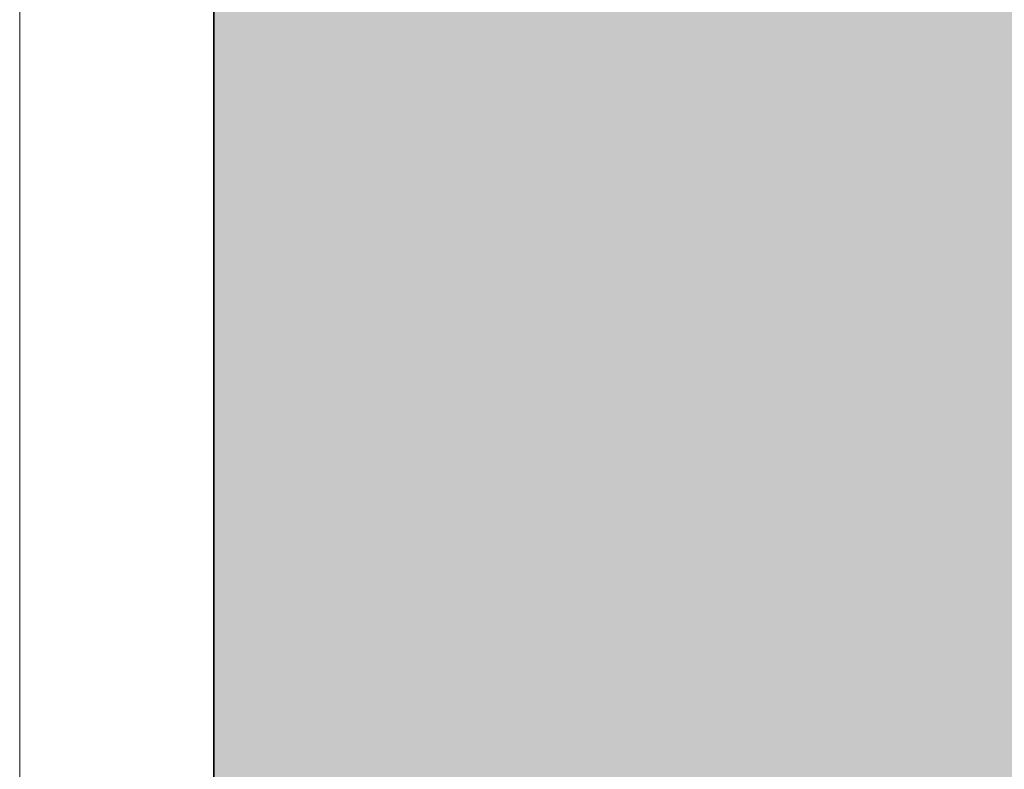
# Model space of a CAD drawing. Units: inches. Extents: x 2091 to 2899, y 967 to 2217.
# Tile 205 of 256: x 2203.1157 to 2203.2571, y 1152.3547 to 1152.4622. Entities that reach past the tile are written whole.
import ezdxf

# ---------------------------------------------------------------- set-up
doc = ezdxf.new("R2010")
doc.units = ezdxf.units.IN
doc.layers.add('A-GLAZ', color=4, linetype='Continuous', lineweight=18)
doc.layers.add('C-PROP', color=7, linetype='Continuous', lineweight=35)
doc.layers.add('A-WALL-PATT', color=141, linetype='Continuous', lineweight=13, true_color=0xadddf7)

# ---------------------------------------------------------------- blocks, each defined once
blk = doc.blocks.new('WIN-DOUBLE-LINE')
blk.add_line((0.0004, -0.00045), (0.0004, 80.8229))

msp = doc.modelspace()

# ---------------------------------------------------------------- hatches: boundary and pattern name
at = {"layer": 'A-WALL-PATT'}
h = msp.add_hatch(color=256, dxfattribs=at)
h.dxf.hatch_style = 1
h.paths.add_polyline_path([(2803.1436, 2050.91906), (2203.1436, 2050.91906), (2203.1436, 1090.91906), (2803.1436, 1090.91906)])
h.paths.add_polyline_path([(2635.79885, 1147.54046), (2674.52405, 1147.54046, 0.376086), (2678.52967, 1152.8802), (2678.52967, 1159.55647, 0.333335), (2674.52432, 1163.56185), (2674.52432, 1163.56185), (2674.52432, 1192.93439), (2635.80597, 1192.93439), (2597.08762, 1192.93439), (2597.08762, 1163.56185, 0.333335), (2593.08228, 1159.55647), (2593.08228, 1152.8802, 0.376086), (2597.08789, 1147.54046)], flags=0)
h.paths.add_polyline_path([(2436.01043, 1278.24078, 0.000483), (2435.95264, 1278.21503, -0.001328), (2435.93563, 1278.11169, -0.001711), (2436.11644, 1278.04076, 0.002185)], flags=0)
h.paths.add_polyline_path([(2794.1436, 1143.41906), (2794.1436, 1347.41906), (2543.37017, 1347.41906), (2543.37017, 1351.91906), (2794.1436, 1351.91906), (2794.1436, 1392.71355), (2793.9474, 1392.71355), (2793.9474, 1473.5369), (2794.1436, 1473.5369), (2794.1436, 1531.91906), (2650.1436, 1531.91906), (2650.1436, 1536.41906), (2794.1436, 1536.41906), (2794.1436, 1692.41906), (2609.37561, 1692.41906), (2609.37561, 1644.41906), (2604.87561, 1644.41906), (2604.87561, 1744.91906), (2609.37561, 1744.91906), (2609.37561, 1696.91906), (2794.1436, 1696.91906), (2794.1436, 1780.91906), (2609.6436, 1780.91906), (2493.87561, 1780.91906), (2493.87561, 1785.41906), (2609.6436, 1785.41906), (2794.1436, 1785.41906), (2794.1436, 1847.93882), (2793.95122, 1847.93882), (2793.95122, 1928.76217), (2794.1436, 1928.76217), (2794.1436, 1941.41906), (2614.1436, 1941.41906), (2614.1436, 1821.41906), (2609.6436, 1821.41906), (2609.6436, 1941.41906), (2392.1436, 1941.41906), (2392.1436, 1819.91906), (2387.6436, 1819.91906), (2387.6436, 1941.41906), (2212.1436, 1941.41906), (2212.1436, 1783.91906), (2392.1436, 1783.91906), (2392.1436, 1780.91906), (2212.1436, 1780.91906), (2212.1436, 1629.41906), (2387.6436, 1629.41906), (2387.6436, 1744.91906), (2392.1436, 1744.91906), (2392.1436, 1627.91906), (2317.1436, 1627.91906), (2317.1436, 1551.41906), (2317.1436, 1536.41906), (2459.38359, 1536.41906), (2459.38359, 1602.39648), (2463.88359, 1602.39648), (2463.88359, 1531.91906), (2456.6436, 1531.91906), (2456.6436, 1529.91906), (2452.1436, 1529.91906), (2452.1436, 1531.91906), (2312.6436, 1531.91906), (2312.6436, 1551.41906), (2306.1436, 1551.41906), (2306.1436, 1555.91906), (2308.1436, 1555.91906), (2308.1436, 1551.41906), (2312.6436, 1551.41906), (2312.6436, 1627.91906), (2212.1436, 1627.91906), (2212.1436, 1555.91906), (2270.1436, 1555.91906), (2270.1436, 1551.41906), (2212.1436, 1551.41906), (2212.1436, 1351.91906), (2272.1436, 1351.91906), (2272.1436, 1347.41906), (2212.1436, 1347.41906), (2212.1436, 1275.41906), (2308.1436, 1275.41906), (2308.1436, 1351.91906), (2452.1436, 1351.91906), (2452.1436, 1493.91906), (2456.6436, 1493.91906), (2456.6436, 1347.41906), (2312.6436, 1347.41906), (2312.6436, 1270.91906), (2212.1436, 1270.91906), (2212.1436, 1099.91906), (2281.23752, 1099.91906), (2282.87104, 1110.9138), (2282.00834, 1116.9966), (2278.55774, 1121.4204), (2268.20564, 1128.0562), (2272.08764, 1128.0562), (2273.81294, 1131.927), (2279.42034, 1134.6919), (2285.02784, 1135.2449), (2287.61584, 1137.4568), (2288.04714, 1138.0098), (2289.34114, 1140.7747), (2291.06654, 1139.6687), (2292.36054, 1135.2449), (2295.37984, 1136.9038), (2296.24254, 1135.7979), (2297.10524, 1133.033), (2300.12464, 1138.0098), (2303.14394, 1138.0098), (2304.43794, 1135.7979), (2303.14394, 1133.586), (2306.59464, 1134.6919), (2307.88874, 1133.033), (2310.90804, 1135.2449), (2313.92744, 1134.1389), (2315.62686, 1132.4271), (2308.32004, 1117.5496), (2290.20384, 1109.8079), (2288.90984, 1103.1721), (2289.27231, 1099.91906), (2434.91823, 1099.91906), (2431.59323, 1124.78806), (2429.93023, 1169.55306), (2430.92718, 1240.51969), (2435.65893, 1238.18613), (2437.13523, 1196.55406), (2438.79823, 1143.97306), (2442.67823, 1111.99806), (2446.55823, 1099.91906), (2794.1436, 1099.91906), (2794.1436, 1138.91906), (2548.03245, 1138.91906), (2548.03245, 1143.41906), (2548.03245, 1148.81906), (2546.66846, 1148.03156), (2528.68569, 1179.17862, 0.256256), (2512.03245, 1148.81906), (2512.03245, 1143.41906), (2512.03245, 1138.91906), (2507.53245, 1138.91906), (2507.53245, 1143.41906), (2507.53245, 1148.81906, 0.256256), (2490.8792, 1179.17862), (2472.89644, 1148.03156), (2471.53245, 1148.81906), (2471.53245, 1143.41906), (2467.03245, 1143.41906), (2467.03245, 1269.94579, 0.039061), (2460.90999, 1273.58006), (2467.03245, 1273.58006), (2467.03245, 1286.32536, 0.014511), (2465.21619, 1286.76191), (2467.03245, 1287.05258), (2467.03245, 1323.41906), (2471.53245, 1323.41906), (2471.53245, 1148.81906), (2489.53245, 1179.99597), (2490.89644, 1179.20847), (2490.8792, 1179.17862, -0.256256), (2507.53245, 1148.81906), (2507.53245, 1143.41906), (2512.03245, 1143.41906), (2512.03245, 1148.81906, -0.256256), (2528.68569, 1179.17862), (2528.66846, 1179.20847), (2530.03245, 1179.99597), (2548.03245, 1148.81906), (2548.03245, 1143.41906)], flags=16)
h.paths.add_polyline_path([(2607.76855, 1200.94508), (2607.76855, 1265.03063), (2597.08762, 1281.05201), (2619.78459, 1281.05201), (2627.79528, 1337.12686), (2635.79885, 1337.12686), (2643.81666, 1337.12686), (2651.82736, 1281.05201), (2674.52432, 1281.05201), (2663.8434, 1265.03063), (2663.8434, 1200.94508), (2635.80597, 1200.94508)], flags=0)
edge = h.paths.add_edge_path(flags=0)
edge.add_ellipse((13303.89622, 1272.99872), major_axis=(-10595.31304, 0), ratio=0.84230387009, start_angle=0.628237219, end_angle=0.6465541, ccw=False)
edge.add_ellipse((2711.70045, 1156.85268), major_axis=(2.21977, 0), ratio=0.8423039, start_angle=111.53524, end_angle=180.62824, ccw=False)
edge.add_ellipse((13303.15629, 1272.99872), major_axis=(-10593.02631, 0), ratio=0.84230386954, start_angle=0.528271472, end_angle=0.646554097, ccw=False)
edge.add_line((2710.7646, 1175.3333), (2710.12999, 1175.3333))
edge.add_ellipse((2710.12999, 1176.57978), major_axis=(1.47985, 0), ratio=0.8423039, start_angle=180, end_angle=270, ccw=False)
edge.add_line((2708.65014, 1176.57978), (2708.65014, 1200.78291))
edge.add_ellipse((2710.12999, 1200.78291), major_axis=(1.47985, 0), ratio=0.8423039, start_angle=90, end_angle=180, ccw=False)
edge.add_line((2710.12999, 1202.02939), (2710.46508, 1202.02939))
edge.add_ellipse((13303.15629, 1272.99872), major_axis=(-10593.02631, 0), ratio=0.84230386954, start_angle=-0.090229089, end_angle=0.383866779, ccw=False)
edge.add_ellipse((2710.12999, 1290.92703), major_axis=(-1.47985, 0), ratio=0.8423039, start_angle=0, end_angle=90, ccw=False)
edge.add_line((2708.65014, 1290.92703), (2708.65014, 1315.13017))
edge.add_ellipse((2710.12999, 1315.13017), major_axis=(-1.47985, 0), ratio=0.8423039, start_angle=-90, end_angle=0, ccw=False)
edge.add_line((2710.12999, 1316.37665), (2710.70631, 1316.37665))
edge.add_ellipse((3238.40172, 1296.28957), major_axis=(528.234, 0), ratio=0.84230387, start_angle=176.3495724, end_angle=177.8200497, ccw=False)
edge.add_ellipse((2775.06304, 1071.4507), major_axis=(313.30776, 0), ratio=0.84230387, start_angle=102.1259656, end_angle=103.780529, ccw=False)
edge.add_ellipse((2775.06304, 1078.3057), major_axis=(-305.30289, 0), ratio=0.84230387, start_angle=-79.790461, end_angle=-77.5553727, ccw=False)
edge.add_ellipse((2695.14177, 1541.97538), major_axis=(-250.96022, 0), ratio=0.84230387, start_angle=99.256566, end_angle=102.5549326)
edge.add_line((2741.41033, 1334.21426), (2747.13255, 1337.37848))
edge.add_ellipse((2747.53862, 1336.85748), major_axis=(-0.73992, 0), ratio=0.842304, start_angle=270, end_angle=307.93313, ccw=False)
edge.add_ellipse((2747.53862, 1336.85748), major_axis=(-0.73992, 0), ratio=0.842304, start_angle=232.06687, end_angle=270, ccw=False)
edge.add_line((2747.94469, 1337.37848), (2753.66691, 1334.21426))
edge.add_ellipse((2799.93547, 1541.97538), major_axis=(250.96022, 0), ratio=0.84230387, start_angle=257.4450674, end_angle=260.743434)
edge.add_ellipse((2720.01419, 1078.3057), major_axis=(305.30289, 0), ratio=0.84230387, start_angle=77.5553727, end_angle=79.790461, ccw=False)
edge.add_ellipse((2720.01419, 1071.4507), major_axis=(-313.30776, 0), ratio=0.84230387, start_angle=256.219471, end_angle=257.8740344, ccw=False)
edge.add_ellipse((2256.67551, 1296.28957), major_axis=(-528.234, 0), ratio=0.84230387, start_angle=182.1799503, end_angle=183.6504276, ccw=False)
edge.add_line((2784.37092, 1316.37665), (2784.94725, 1316.37665))
edge.add_ellipse((2784.94725, 1315.13017), major_axis=(1.47985, 0), ratio=0.8423039, start_angle=0, end_angle=90, ccw=False)
edge.add_line((2786.42709, 1315.13017), (2786.42709, 1290.92703))
edge.add_ellipse((2784.94725, 1290.92703), major_axis=(1.47985, 0), ratio=0.8423039, start_angle=270, end_angle=360, ccw=False)
edge.add_ellipse((-7808.07906, 1272.99872), major_axis=(10593.02631, 0), ratio=0.84230386954, start_angle=-0.383866779, end_angle=0.090229089, ccw=False)
edge.add_line((2784.61216, 1202.02939), (2784.94725, 1202.02939))
edge.add_ellipse((2784.94725, 1200.78291), major_axis=(1.47985, 0), ratio=0.8423039, start_angle=0, end_angle=90, ccw=False)
edge.add_line((2786.42709, 1200.78291), (2786.42709, 1176.57978))
edge.add_ellipse((2784.94725, 1176.57978), major_axis=(-1.47985, 0), ratio=0.8423039, start_angle=90, end_angle=180, ccw=False)
edge.add_line((2784.94725, 1175.3333), (2784.31264, 1175.3333))
edge.add_ellipse((-7808.07906, 1272.99872), major_axis=(10593.02631, 0), ratio=0.84230386954, start_angle=-0.618643196, end_angle=-0.528271472, ccw=False)
edge.add_ellipse((2783.37678, 1156.85268), major_axis=(-2.21977, 0), ratio=0.8423039, start_angle=179.37176, end_angle=248.46476, ccw=False)
edge.add_ellipse((-7808.81898, 1272.99872), major_axis=(-10595.31304, 0), ratio=0.84230386576, start_angle=179.353445923, end_angle=179.371762803, ccw=False)
edge.add_ellipse((2780.2973, 1153.50079), major_axis=(-5.24643, 0), ratio=0.8423039, start_angle=90, end_angle=179.35345, ccw=False)
edge.add_line((2780.2973, 1149.08171), (2714.77993, 1149.08171))
edge.add_ellipse((2714.77993, 1153.50079), major_axis=(5.24643, 0), ratio=0.8423039, start_angle=180.64655, end_angle=270, ccw=False)
edge = h.paths.add_edge_path(flags=0)
edge.add_line((2718.18737, 1151.00783), (2718.18737, 1170.47236))
edge.add_ellipse((2721.14706, 1170.47236), major_axis=(-2.95969, 0), ratio=0.8423039, start_angle=-90, end_angle=0, ccw=False)
edge.add_line((2721.14706, 1172.96532), (2773.93017, 1172.96532))
edge.add_ellipse((2773.93017, 1170.47236), major_axis=(-2.95969, 0), ratio=0.8423039, start_angle=180, end_angle=270, ccw=False)
edge.add_line((2776.88987, 1170.47236), (2776.88987, 1151.00783))
edge.add_line((2776.88987, 1151.00783), (2718.18737, 1151.00783))
edge = h.paths.add_edge_path(flags=0)
edge.add_line((2718.18737, 1180.23415), (2718.18737, 1199.05783))
edge.add_ellipse((2747.53862, 1320.39864), major_axis=(147.01792, 0), ratio=0.84230387, start_angle=256.4018653, end_angle=283.5981347)
edge.add_line((2776.88987, 1199.05783), (2776.88987, 1180.23415))
edge.add_ellipse((2747.53862, 1301.57496), major_axis=(147.01792, 0), ratio=0.84230387, start_angle=256.4018653, end_angle=283.5981347, ccw=False)
edge = h.paths.add_edge_path(flags=0)
edge.add_ellipse((13303.15629, 1272.99872), major_axis=(-10591.54646, 0), ratio=0.84230386955, start_angle=0.055594314, end_angle=0.377764194, ccw=False)
edge.add_line((2711.61686, 1262.72171), (2715.66741, 1249.4954))
edge.add_ellipse((6413.89196, 1241.69192), major_axis=(-3698.23616, 0), ratio=0.8423038695, start_angle=-0.12089737, end_angle=0.36407635)
edge.add_line((2715.76104, 1218.19245), (2711.93431, 1203.16736))
edge = h.paths.add_edge_path(flags=0)
edge.add_line((2718.18737, 1251.07457), (2716.00249, 1267.45044))
edge.add_ellipse((2742.15117, 1202.18954), major_axis=(81.77258, 0), ratio=0.84230387, start_angle=94.277421, end_angle=111.8349538, ccw=False)
edge.add_line((2737.00975, 1270.93063), (2758.06748, 1270.93063))
edge.add_ellipse((2752.92606, 1202.18954), major_axis=(81.77258, 0), ratio=0.84230387, start_angle=68.1650462, end_angle=85.722579, ccw=False)
edge.add_line((2779.07475, 1267.45044), (2776.88987, 1251.07457))
edge.add_ellipse((2750.33806, 1187.88536), major_axis=(79.57966, 0), ratio=0.84230387, start_angle=67.2080851, end_angle=85.1299304)
edge.add_line((2756.03466, 1254.74366), (2739.04258, 1254.74366))
edge.add_ellipse((2744.73917, 1187.88536), major_axis=(79.57966, 0), ratio=0.84230387, start_angle=94.8700696, end_angle=112.7919149)
edge = h.paths.add_edge_path(flags=0)
edge.add_line((2783.14293, 1203.16736), (2779.31619, 1218.19245))
edge.add_ellipse((-918.81473, 1241.69192), major_axis=(3698.23616, 0), ratio=0.8423038695, start_angle=-0.36407635, end_angle=0.12089737)
edge.add_line((2779.40983, 1249.4954), (2783.46037, 1262.72171))
edge.add_ellipse((-7808.07906, 1272.99872), major_axis=(-10591.54646, 0), ratio=0.84230386954, start_angle=179.622235806, end_angle=179.944405687, ccw=False)
edge = h.paths.add_edge_path(flags=0)
edge.add_ellipse((2734.20089, 1286.69044), major_axis=(-0.35661, 6.34008), ratio=0.6038336, start_angle=89.002014, end_angle=253.657408, ccw=False)
edge.add_line((2730.369, 1286.54181), (2730.369, 1301.35198))
edge.add_line((2730.369, 1301.35198), (2735.91331, 1305.2148))
edge.add_ellipse((2736.38492, 1304.73456), major_axis=(0.73992, 0), ratio=0.842304, start_angle=90, end_angle=134.48021, ccw=False)
edge.add_line((2736.38492, 1305.3578), (2738.03278, 1305.3578))
edge.add_line((2738.03278, 1305.3578), (2738.03278, 1307.70793))
edge.add_ellipse((2794.20164, 1307.70793), major_axis=(56.16886, 0), ratio=0.84230387, start_angle=150.56143, end_angle=180, ccw=False)
edge.add_ellipse((2700.87559, 1307.70793), major_axis=(-56.16886, 0), ratio=0.84230387, start_angle=180, end_angle=209.43857, ccw=False)
edge.add_line((2757.04445, 1307.70793), (2757.04445, 1305.3578))
edge.add_line((2757.04445, 1305.3578), (2758.69232, 1305.3578))
edge.add_ellipse((2758.69232, 1304.73456), major_axis=(-0.73992, 0), ratio=0.842304, start_angle=225.51979, end_angle=270, ccw=False)
edge.add_line((2759.16392, 1305.2148), (2764.70823, 1301.35198))
edge.add_line((2764.70823, 1301.35198), (2764.70823, 1286.54181))
edge.add_ellipse((2760.87634, 1286.69044), major_axis=(0.35661, 6.34008), ratio=0.6038336, start_angle=106.342592, end_angle=270.997986, ccw=False)
edge.add_line((2757.04445, 1285.79709), (2757.04445, 1307.70793))
edge.add_ellipse((2700.87559, 1307.70793), major_axis=(-56.16886, 0), ratio=0.84230387, start_angle=180, end_angle=209.43857)
edge.add_ellipse((2794.20164, 1307.70793), major_axis=(56.16886, 0), ratio=0.84230387, start_angle=150.56143, end_angle=180)
edge.add_line((2738.03278, 1307.70793), (2738.03278, 1285.79709))
h.paths.add_polyline_path([(2417.81227, 1104.4497), (2413.49227, 1102.5297), (2410.61227, 1103.9697), (2409.17227, 1106.3697), (2407.25227, 1107.3297), (2406.29227, 1109.7297), (2405.33227, 1114.0497), (2405.33227, 1117.8897), (2406.29227, 1120.1297), (2407.25227, 1119.8097), (2408.84832, 1118.32766), (2410.17395, 1119.42417), (2410.21127, 1120.4057), (2411.04073, 1121.41905), (2410.69927, 1119.8587), (2410.17395, 1119.42417), (2410.08845, 1117.17611), (2411.13284, 1116.20632), (2413.97227, 1119.3297), (2416.85227, 1120.7697), (2416.86972, 1120.79878), (2417.03507, 1119.40512), (2417.89621, 1118.14338), (2418.29227, 1118.3697), (2419.54445, 1120.03927), (2419.36092, 1118.38749), (2419.03211, 1119.35615), (2418.39894, 1118.51193), (2419.25227, 1114.5297), (2418.79409, 1107.19879)], flags=0)
h.paths.add_polyline_path([(2508.87017, 1347.41906), (2508.37017, 1347.41906), (2508.37017, 1351.91906), (2508.87017, 1351.91906)], flags=0)
h.paths.add_polyline_path([(2473.37017, 1347.41906), (2472.37017, 1347.41906), (2467.87017, 1347.41906), (2467.87017, 1455.41906), (2472.37017, 1455.41906), (2472.37017, 1352.41906), (2473.37017, 1352.41906)], flags=0)
h.paths.add_polyline_path([(2352.10624, 1217.4462), (2349.22624, 1218.8862), (2347.78624, 1221.2862), (2345.86624, 1222.2462), (2344.90624, 1224.6462), (2343.94624, 1228.9662), (2343.94624, 1232.8062), (2344.90624, 1235.0462), (2345.86624, 1234.7262), (2347.46229, 1233.24415), (2348.78792, 1234.34066), (2348.82524, 1235.3222), (2349.6547, 1236.33555), (2349.31324, 1234.7752), (2348.78792, 1234.34066), (2348.70242, 1232.0926), (2349.74681, 1231.12282), (2352.58624, 1234.2462), (2355.46624, 1235.6862), (2355.48369, 1235.71528), (2355.64904, 1234.32161), (2356.51018, 1233.05988), (2356.90624, 1233.2862), (2358.15842, 1234.95576), (2357.97489, 1233.30398), (2357.64608, 1234.27264), (2357.01291, 1233.42842), (2357.86624, 1229.4462), (2357.40806, 1222.11529), (2356.42624, 1219.3662)], flags=0)
h.paths.add_polyline_path([(2348.2968, 1112.22442), (2347.0138, 1112.31042), (2345.5298, 1114.12742), (2345.7318, 1115.85842), (2346.8118, 1116.98242), (2346.8118, 1114.64642), (2345.8668, 1114.21442), (2346.8798, 1114.30042)], flags=0)
h.paths.add_polyline_path([(2347.0138, 1110.92642), (2346.2718, 1110.49342), (2346.6098, 1111.18642)], flags=0)
h.paths.add_polyline_path([(2345.8668, 1118.19442), (2345.5298, 1117.32942), (2343.7078, 1118.02142), (2344.3828, 1118.62642)], flags=0)
h.paths.add_polyline_path([(2346.6768, 1109.28242), (2346.0698, 1108.07142), (2345.8668, 1110.06142)], flags=0)
h.paths.add_polyline_path([(2345.0568, 1119.75142), (2343.6398, 1119.75142), (2343.9778, 1121.13542)], flags=0)
h.paths.add_polyline_path([(2345.2598, 1116.55042), (2345.1248, 1115.85842), (2344.9218, 1115.68542), (2344.7198, 1116.37742)], flags=0)
h.paths.add_polyline_path([(2345.6648, 1112.31042), (2345.4618, 1111.53242), (2344.0448, 1111.96442), (2344.6518, 1112.57042)], flags=0)
h.paths.add_polyline_path([(2345.1918, 1113.34942), (2344.4498, 1113.86842), (2344.7198, 1114.38742)], flags=0)
h.paths.add_polyline_path([(2344.6518, 1116.80942), (2344.1798, 1115.68542), (2344.6518, 1115.33942), (2343.9098, 1114.90642), (2343.0328, 1115.94442), (2343.6398, 1116.46342)], flags=0)
h.paths.add_polyline_path([(2345.8668, 1106.68642), (2344.9898, 1105.56242), (2344.5168, 1106.60042)], flags=0)
h.paths.add_polyline_path([(2344.8548, 1110.06142), (2344.5168, 1109.28242), (2344.1128, 1109.71542)], flags=0)
h.paths.add_polyline_path([(2344.0448, 1113.52242), (2343.4378, 1113.08942), (2342.7628, 1113.95442)], flags=0)
h.paths.add_polyline_path([(2344.3148, 1111.01242), (2342.9648, 1110.32042), (2342.9648, 1111.09942)], flags=0)
h.paths.add_polyline_path([(2345.1248, 1104.69742), (2344.5848, 1103.74542), (2344.4498, 1104.26442)], flags=0)
h.paths.add_polyline_path([(2342.8298, 1121.22242), (2341.7498, 1120.53042), (2340.5358, 1121.04942), (2340.1308, 1121.82842), (2340.6708, 1122.95242), (2341.1428, 1121.82842), (2341.6148, 1122.00142)], flags=0)
h.paths.add_polyline_path([(2342.9648, 1119.75142), (2343.0328, 1118.45342), (2342.0878, 1118.02142), (2342.0198, 1119.49142)], flags=0)
h.paths.add_polyline_path([(2342.6948, 1116.89642), (2341.9528, 1116.63642), (2342.0198, 1117.32942)], flags=0)
h.paths.add_polyline_path([(2343.0328, 1112.22442), (2342.0198, 1111.79142), (2341.5478, 1112.22442), (2342.3578, 1113.34942)], flags=0)
h.paths.add_polyline_path([(2343.7748, 1104.43742), (2342.6278, 1102.88042), (2342.6948, 1104.61042), (2343.4378, 1105.12942)], flags=0)
h.paths.add_polyline_path([(2342.0198, 1115.07942), (2340.8058, 1115.51242), (2340.9408, 1116.37742)], flags=0)
h.paths.add_polyline_path([(2341.4808, 1120.09742), (2341.4808, 1119.40542), (2341.0758, 1119.57842), (2341.1428, 1120.09742)], flags=0)
h.paths.add_polyline_path([(2341.8178, 1114.47342), (2340.9408, 1113.08942), (2340.8058, 1114.56042)], flags=0)
h.paths.add_polyline_path([(2341.1428, 1118.54042), (2340.9408, 1116.98242), (2339.0508, 1117.67542), (2339.0508, 1118.62642)], flags=0)
h.paths.add_polyline_path([(2342.6948, 1101.66842), (2341.9528, 1101.84142), (2342.5598, 1102.36142)], flags=0)
h.paths.add_polyline_path([(2340.3328, 1119.66542), (2338.4438, 1119.57842), (2337.9038, 1120.35742), (2339.6578, 1120.61642)], flags=0)
h.paths.add_polyline_path([(2340.3328, 1115.33942), (2340.0628, 1113.69542), (2339.3878, 1115.33942)], flags=0)
h.paths.add_polyline_path([(2341.8178, 1103.83142), (2341.5478, 1102.88042), (2341.1428, 1103.65842)], flags=0)
h.paths.add_polyline_path([(2339.0508, 1122.86642), (2337.2958, 1121.82842), (2337.0938, 1123.12542), (2337.7688, 1123.81842)], flags=0)
h.paths.add_polyline_path([(2339.1178, 1121.74142), (2338.8478, 1121.22242), (2338.1738, 1121.04942), (2338.3758, 1121.56842)], flags=0)
h.paths.add_polyline_path([(2339.1858, 1119.31942), (2338.6458, 1118.71342), (2338.2408, 1118.10742), (2338.2408, 1118.88642)], flags=0)
h.paths.add_polyline_path([(2341.1428, 1101.92842), (2340.6028, 1101.23642), (2340.0628, 1101.84142), (2340.6028, 1102.36142)], flags=0)
h.paths.add_polyline_path([(2337.6338, 1117.76142), (2336.6208, 1118.28042), (2337.2958, 1118.97242)], flags=0)
h.paths.add_polyline_path([(2336.8238, 1119.57842), (2334.7988, 1118.97242), (2335.2038, 1120.35742), (2336.5538, 1120.87642)], flags=0)
h.paths.add_polyline_path([(2339.1178, 1100.45742), (2337.3638, 1100.54342), (2336.7558, 1101.23642)], flags=0)
h.paths.add_polyline_path([(2336.3508, 1122.43342), (2336.0138, 1121.91442), (2334.9338, 1122.43342), (2334.5288, 1123.47142), (2335.7438, 1122.77942)], flags=0)
h.paths.add_polyline_path([(2334.7318, 1120.87642), (2334.2588, 1120.35742), (2334.0568, 1120.78942), (2334.5968, 1121.30842)], flags=0)
h.paths.add_polyline_path([(2334.4618, 1122.17442), (2332.5718, 1121.30842), (2331.3568, 1122.17442), (2332.0998, 1122.86642)], flags=0)
h.paths.add_polyline_path([(2334.2588, 1118.54042), (2333.3818, 1118.45342), (2333.6518, 1119.31942)], flags=0)
h.paths.add_polyline_path([(2335.5418, 1102.27442), (2334.1918, 1102.62042), (2335.2718, 1103.31242)], flags=0)
h.paths.add_polyline_path([(2332.7068, 1119.66542), (2331.6948, 1120.44342), (2332.5048, 1120.78942)], flags=0)
h.paths.add_polyline_path([(2334.7318, 1101.14942), (2333.5168, 1101.58242), (2333.9888, 1101.75542)], flags=0)
h.paths.add_polyline_path([(2332.6398, 1116.63642), (2331.0868, 1116.29042), (2331.9648, 1118.19442)], flags=0)
h.paths.add_polyline_path([(2330.7498, 1121.56842), (2330.2768, 1120.27042), (2328.5228, 1119.31942), (2328.9948, 1121.04942)], flags=0)
h.paths.add_polyline_path([(2330.7498, 1118.62642), (2330.0078, 1117.50242), (2329.8728, 1118.02142)], flags=0)
h.paths.add_polyline_path([(2332.0998, 1102.36142), (2330.5468, 1102.01442), (2331.6948, 1102.96642)], flags=0)
h.paths.add_polyline_path([(2329.5348, 1113.60842), (2329.0628, 1112.31042), (2328.5898, 1113.34942)], flags=0)
h.paths.add_polyline_path([(2328.3878, 1117.84842), (2327.5098, 1116.55042), (2327.1728, 1117.76142)], flags=0)
h.paths.add_polyline_path([(2329.7378, 1106.51342), (2329.5348, 1105.30242), (2328.2528, 1106.08142)], flags=0)
h.paths.add_polyline_path([(2328.6578, 1114.38742), (2328.0498, 1114.12742), (2328.3198, 1114.90642)], flags=0)
h.paths.add_polyline_path([(2328.3198, 1112.22442), (2327.1058, 1112.13742), (2326.7008, 1112.65642)], flags=0)
h.paths.add_polyline_path([(2326.9028, 1115.25242), (2326.7008, 1114.12742), (2325.2158, 1113.60842), (2326.0928, 1115.33942)], flags=0)
h.paths.add_polyline_path([(2326.6328, 1108.33042), (2326.0928, 1107.37942), (2325.8908, 1108.50342), (2326.4978, 1109.10942)], flags=0)
h.paths.add_polyline_path([(2615.1436, 1531.91906), (2609.6436, 1531.91906), (2609.6436, 1620.41906), (2614.1436, 1620.41906), (2614.1436, 1536.41906), (2615.1436, 1536.41906)], flags=0)
h.paths.add_polyline_path([(2545.1436, 1563.41906), (2464.1436, 1563.41906), (2464.1436, 1632.41906), (2509.1436, 1632.41906), (2509.1436, 1627.91906), (2509.1436, 1603.91906), (2468.6436, 1603.91906), (2468.6436, 1567.91906), (2540.6436, 1567.91906), (2540.6436, 1591.91906), (2545.1436, 1591.91906)], flags=0)
h.paths.add_polyline_path([(2388.96905, 1549.98573), (2357.43418, 1549.98573), (2357.43418, 1623.36078), (2399.36278, 1623.36078), (2435.68947, 1623.36078), (2435.59255, 1602.55927), (2435.59255, 1602.39648), (2388.96905, 1602.39648)], flags=0)
h.paths.add_polyline_path([(2388.88063, 1555.80915), (2374.90443, 1555.80915), (2374.90443, 1600.57156), (2374.90443, 1615.45765), (2406.35088, 1615.45765), (2406.35088, 1618.93943), (2412.17429, 1615.45765), (2406.35088, 1611.97586), (2406.35088, 1615.45765), (2388.88063, 1615.45765)], flags=0)
h.paths.add_polyline_path([(2568.87561, 1644.41906), (2453.37561, 1644.41906), (2453.37561, 1785.41906), (2457.87561, 1785.41906), (2457.87561, 1648.91906), (2568.87561, 1648.91906)], flags=0)
h.paths.add_polyline_path([(2212.1436, 1945.91906), (2212.1436, 2041.91906), (2794.1436, 2041.91906), (2794.1436, 1945.91906)], flags=16)
h.paths.add_polyline_path([(2271.08273, 1964.31724), (2776.85297, 1964.31724), (2776.85297, 2037.16962), (2271.08273, 2037.16962)], flags=8)
h.paths.add_polyline_path([(2380.64929, 1536.82414), (2461.04081, 1536.82414), (2461.04081, 1554.65259), (2380.64929, 1554.65259)], flags=8)
h.paths.add_polyline_path([(2240.75571, 1609.72545), (2309.18583, 1609.72545), (2309.18583, 1617.6982), (2240.75571, 1617.6982)], flags=8)
h.paths.add_polyline_path([(2212.67726, 1313.5041), (2282.59152, 1313.5041), (2282.59152, 1322.74524), (2212.67726, 1322.74524)], flags=8)
h.paths.add_polyline_path([(2457.11198, 1114.77857), (2558.48158, 1114.77857), (2558.48158, 1142.21968), (2457.11198, 1142.21968)], flags=8)
h.paths.add_polyline_path([(2473.44234, 1273.01007), (2604.64123, 1273.01007), (2604.64123, 1318.34693), (2473.44234, 1318.34693)], flags=8)
h.paths.add_polyline_path([(2638.8763, 1626.97743), (2684.25037, 1627.97674), (2684.03848, 1637.59749), (2638.66442, 1636.59819)], flags=8)
h.paths.add_polyline_path([(2537.59055, 1453.79345), (2628.38955, 1453.79345), (2628.38955, 1475.34481), (2537.59055, 1475.34481)], flags=8)
h.paths.add_polyline_path([(2504.13764, 1714.6324), (2554.64719, 1714.6324), (2554.64719, 1730.23771), (2504.13764, 1730.23771)], flags=8)
h.paths.add_polyline_path([(2487.50118, 1575.65187), (2535.09712, 1575.65187), (2535.09712, 1598.37765), (2487.50118, 1598.37765)], flags=8)
h.paths.add_polyline_path([(2709.0994, 1735.71028), (2740.0166, 1735.71028), (2740.0166, 1749.93764), (2709.0994, 1749.93764)], flags=8)
h.paths.add_polyline_path([(2442.43842, 1792.17166), (2564.72884, 1792.17166), (2564.72884, 1842.00016), (2442.43842, 1842.00016)], flags=8)
h.paths.add_polyline_path([(2655.8158, 1809.64408), (2789.52014, 1806.6938), (2790.08498, 1832.29164), (2656.38064, 1835.24192)], flags=8)
h.paths.add_polyline_path([(2234.8427, 1797.72014), (2368.59285, 1794.76885), (2369.16072, 1820.50413), (2235.41056, 1823.45542)], flags=8)
h.paths.add_polyline_path([(2245.13847, 1644.00633), (2398.42773, 1640.6239), (2398.99484, 1666.32482), (2245.70557, 1669.70725)], flags=8)
h.paths.add_polyline_path([(2306.14285, 1431.16852), (2413.76831, 1428.79369), (2414.33315, 1454.39153), (2306.70768, 1456.76636)], flags=8)
h.paths.add_polyline_path([(2306.83458, 1458.23314), (2393.38048, 1456.32345), (2393.93281, 1481.35436), (2307.38691, 1483.26405)], flags=8)

# ---------------------------------------------------------------- linework, layer by layer
at = {"layer": 'C-PROP'}
msp.add_lwpolyline([(2203.1436, 2050.91906), (2803.1436, 2050.91906), (2803.1436, 1090.91906), (2203.1436, 1090.91906)], close=True, dxfattribs=at)

# ---------------------------------------------------------------- block references
at = {"layer": 'A-GLAZ'}
msp.add_blockref('WIN-DOUBLE-LINE', (2203.11534, 1152.2475), dxfattribs=at)

doc.saveas('drawing.dxf')
